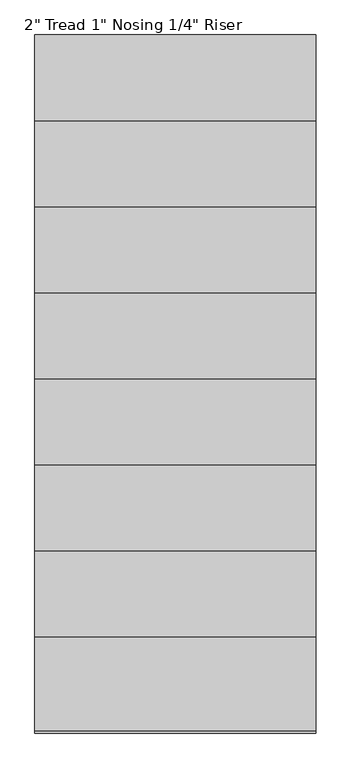
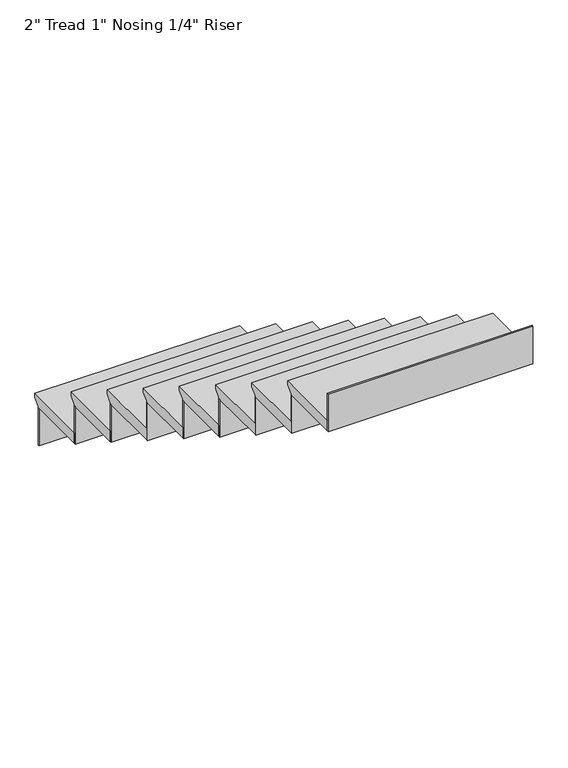
"""IFC4 building model written with IfcOpenShell, lengths in millimetres: stair flight geometry."""

from ifc_helpers import new_model, si_unit, frame, origin, place, context, project, spatial, polyline, outline, extrude, source, transform, mapped, element, save


def stair_flight_0c18b218(model_context):
    return source(origin(), model_context, "Body", "SweptSolid", [
        extrude(outline(polyline([(8107.643496, 8788.4), (8412.443496, 8788.4), (8412.443496, 8769.35), (8387.043496, 8743.95), (8387.043496, 8737.6), (8107.643496, 8737.6), (8107.643496, 8788.4)])), frame((-11538.468339, 0.0, 0.0), z_axis=(1.0, 0.0, 0.0), x_axis=(0.0, 1.0, 0.0)), (0.0, 0.0, 1.0), 914.4),
        extrude(outline(polyline([(-11538.468339, 8380.693496), (-11538.468339, 8387.043496), (-10624.068339, 8387.043496), (-10624.068339, 8380.693496), (-11538.468339, 8380.693496)])), frame((0.0, 0.0, 8559.8), z_axis=(0.0, 0.0, 1.0), x_axis=(1.0, 0.0, 0.0)), (0.0, 0.0, 1.0), 177.8),
        extrude(outline(polyline([(-11538.468339, 8101.293496), (-11538.468339, 8107.643496), (-10624.068339, 8107.643496), (-10624.068339, 8101.293496), (-11538.468339, 8101.293496)])), frame((0.0, 0.0, 8737.6), z_axis=(0.0, 0.0, 1.0), x_axis=(1.0, 0.0, 0.0)), (0.0, 0.0, 1.0), 177.8),
        extrude(outline(polyline([(7828.243496, 8966.2), (8133.043496, 8966.2), (8133.043496, 8947.15), (8107.643496, 8921.75), (8107.643496, 8915.4), (7828.243496, 8915.4), (7828.243496, 8966.2)])), frame((-11538.468339, 0.0, 0.0), z_axis=(1.0, 0.0, 0.0), x_axis=(0.0, 1.0, 0.0)), (0.0, 0.0, 1.0), 914.4),
        extrude(outline(polyline([(-11538.468339, 7821.893496), (-11538.468339, 7828.243496), (-10624.068339, 7828.243496), (-10624.068339, 7821.893496), (-11538.468339, 7821.893496)])), frame((0.0, 0.0, 8915.4), z_axis=(0.0, 0.0, 1.0), x_axis=(1.0, 0.0, 0.0)), (0.0, 0.0, 1.0), 177.8),
        extrude(outline(polyline([(7548.843496, 9144.0), (7853.643496, 9144.0), (7853.643496, 9124.95), (7828.243496, 9099.55), (7828.243496, 9093.2), (7548.843496, 9093.2), (7548.843496, 9144.0)])), frame((-11538.468339, 0.0, 0.0), z_axis=(1.0, 0.0, 0.0), x_axis=(0.0, 1.0, 0.0)), (0.0, 0.0, 1.0), 914.4),
        extrude(outline(polyline([(-11538.468339, 7542.493496), (-11538.468339, 7548.843496), (-10624.068339, 7548.843496), (-10624.068339, 7542.493496), (-11538.468339, 7542.493496)])), frame((0.0, 0.0, 9093.2), z_axis=(0.0, 0.0, 1.0), x_axis=(1.0, 0.0, 0.0)), (0.0, 0.0, 1.0), 177.8),
        extrude(outline(polyline([(7269.443496, 9321.8), (7574.243496, 9321.8), (7574.243496, 9302.75), (7548.843496, 9277.35), (7548.843496, 9271.0), (7269.443496, 9271.0), (7269.443496, 9321.8)])), frame((-11538.468339, 0.0, 0.0), z_axis=(1.0, 0.0, 0.0), x_axis=(0.0, 1.0, 0.0)), (0.0, 0.0, 1.0), 914.4),
        extrude(outline(polyline([(-11538.468339, 7263.093496), (-11538.468339, 7269.443496), (-10624.068339, 7269.443496), (-10624.068339, 7263.093496), (-11538.468339, 7263.093496)])), frame((0.0, 0.0, 9271.0), z_axis=(0.0, 0.0, 1.0), x_axis=(1.0, 0.0, 0.0)), (0.0, 0.0, 1.0), 177.8),
        extrude(outline(polyline([(6990.043496, 9499.6), (7294.843496, 9499.6), (7294.843496, 9480.55), (7269.443496, 9455.15), (7269.443496, 9448.8), (6990.043496, 9448.8), (6990.043496, 9499.6)])), frame((-11538.468339, 0.0, 0.0), z_axis=(1.0, 0.0, 0.0), x_axis=(0.0, 1.0, 0.0)), (0.0, 0.0, 1.0), 914.4),
        extrude(outline(polyline([(-11538.468339, 6983.693496), (-11538.468339, 6990.043496), (-10624.068339, 6990.043496), (-10624.068339, 6983.693496), (-11538.468339, 6983.693496)])), frame((0.0, 0.0, 9448.8), z_axis=(0.0, 0.0, 1.0), x_axis=(1.0, 0.0, 0.0)), (0.0, 0.0, 1.0), 177.8),
        extrude(outline(polyline([(6710.643496, 9677.4), (7015.443496, 9677.4), (7015.443496, 9658.35), (6990.043496, 9632.95), (6990.043496, 9626.6), (6710.643496, 9626.6), (6710.643496, 9677.4)])), frame((-11538.468339, 0.0, 0.0), z_axis=(1.0, 0.0, 0.0), x_axis=(0.0, 1.0, 0.0)), (0.0, 0.0, 1.0), 914.4),
        extrude(outline(polyline([(-11538.468339, 6704.293496), (-11538.468339, 6710.643496), (-10624.068339, 6710.643496), (-10624.068339, 6704.293496), (-11538.468339, 6704.293496)])), frame((0.0, 0.0, 9626.6), z_axis=(0.0, 0.0, 1.0), x_axis=(1.0, 0.0, 0.0)), (0.0, 0.0, 1.0), 177.8),
        extrude(outline(polyline([(6431.243496, 9855.2), (6736.043496, 9855.2), (6736.043496, 9836.15), (6710.643496, 9810.75), (6710.643496, 9804.4), (6431.243496, 9804.4), (6431.243496, 9855.2)])), frame((-11538.468339, 0.0, 0.0), z_axis=(1.0, 0.0, 0.0), x_axis=(0.0, 1.0, 0.0)), (0.0, 0.0, 1.0), 914.4),
        extrude(outline(polyline([(-11538.468339, 6424.893496), (-11538.468339, 6431.243496), (-10624.068339, 6431.243496), (-10624.068339, 6424.893496), (-11538.468339, 6424.893496)])), frame((0.0, 0.0, 9804.4), z_axis=(0.0, 0.0, 1.0), x_axis=(1.0, 0.0, 0.0)), (0.0, 0.0, 1.0), 177.8),
        extrude(outline(polyline([(-11538.468339, 6145.493496), (-11538.468339, 6151.843496), (-10624.068339, 6151.843496), (-10624.068339, 6145.493496), (-11538.468339, 6145.493496)])), frame((0.0, 0.0, 9982.2), z_axis=(0.0, 0.0, 1.0), x_axis=(1.0, 0.0, 0.0)), (0.0, 0.0, 1.0), 177.8),
        extrude(outline(polyline([(6151.843496, 10033.0), (6456.643496, 10033.0), (6456.643496, 10013.95), (6431.243496, 9988.55), (6431.243496, 9982.2), (6151.843496, 9982.2), (6151.843496, 10033.0)])), frame((-11538.468339, 0.0, 0.0), z_axis=(1.0, 0.0, 0.0), x_axis=(0.0, 1.0, 0.0)), (0.0, 0.0, 1.0), 914.4),
    ])


if __name__ == "__main__":
    model = new_model("IFC4")
    model_context = context("Model", 3, world=origin())
    ifc_project = project(units=[si_unit("LENGTHUNIT", "METRE", prefix="MILLI")], contexts=[model_context])
    site = spatial("IfcSite", under=ifc_project)
    building = spatial("IfcBuilding", under=site)
    placement = place(None, origin())
    stair_flight_shape = stair_flight_0c18b218(model_context)
    element("IfcStairFlight", 1, ObjectType="2\" Tread 1\" Nosing 1/4\" Riser", at=placement, inside=building, context=model_context, shape_type="MappedRepresentation", body=[
        mapped(stair_flight_shape, transform((0.0, 0.0, 0.0), x_axis=(1.0, 0.0, 0.0), y_axis=(0.0, 1.0, 0.0), z_axis=(0.0, 0.0, 1.0))),
    ])
    save(model, "model.ifc")
